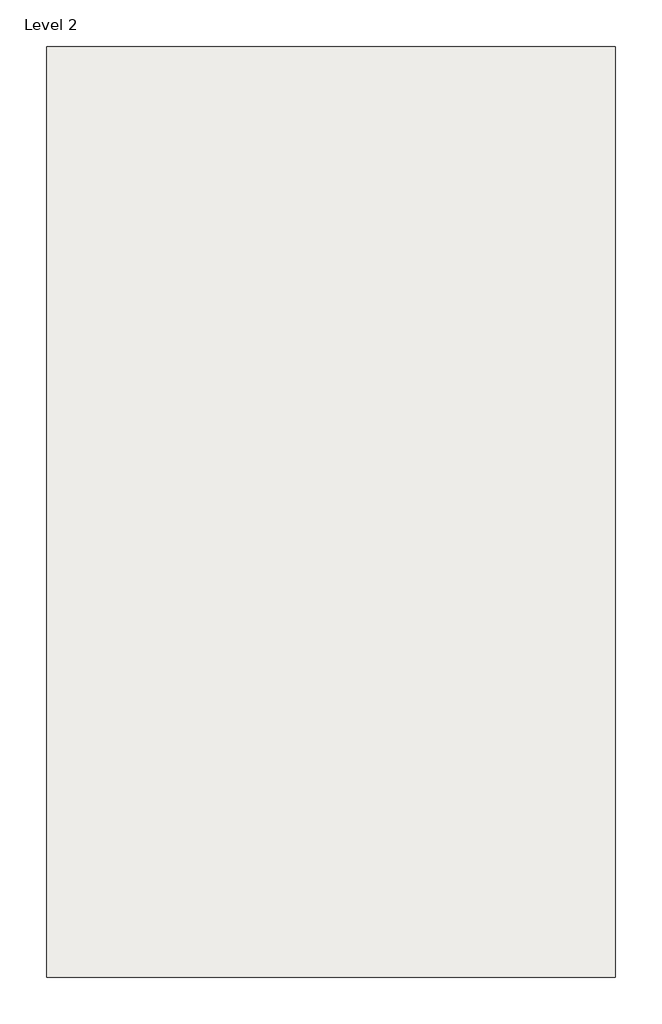
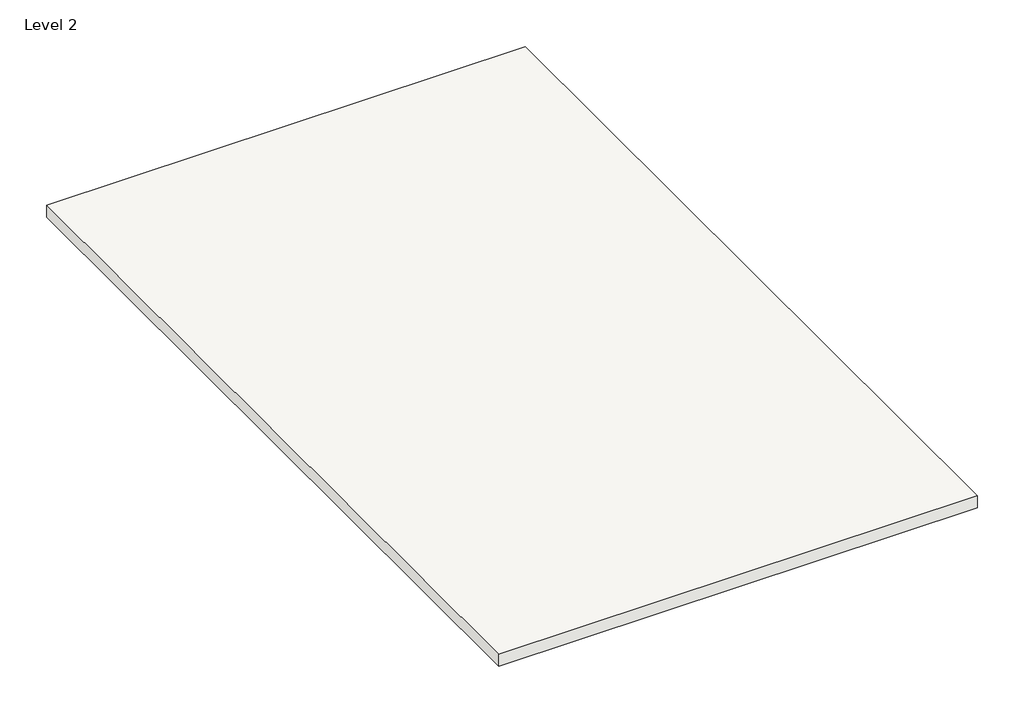
# One storey: 1 roof.
"""IFC4 building model written with IfcOpenShell, lengths in millimetres."""

from ifc_helpers import new_model, si_unit, frame, origin, place, context, project, spatial, polyline, outline, extrude, element, save

model = new_model("IFC4")

# Units and contexts
model_context = context("Model", 3, world=origin())
ifc_project = project(units=[si_unit("LENGTHUNIT", "METRE", prefix="MILLI")], contexts=[model_context])

# Site, building, storey
site = spatial("IfcSite", under=ifc_project)
building = spatial("IfcBuilding", under=site)
storey = spatial("IfcBuildingStorey", under=building, Name="Level 2", Elevation=3048.0)

# Roof
placement = place(None, origin())
element("IfcRoof", 1, ObjectType="Generic - 12\"", at=placement, inside=storey, context=model_context, shape_type="SweptSolid", body=[
    extrude(outline(polyline([(-12835.5505662, 12819.7742707), (-1354.7505662, 12819.7742707), (-1354.7505662, -5976.2257293), (-12835.5505662, -5976.2257293), (-12835.5505662, 12819.7742707)])), frame((0.0, 0.0, 3048.0), z_axis=(0.0, 0.0, 1.0), x_axis=(1.0, 0.0, 0.0)), (0.0, 0.0, 1.0), 304.8),
])

save(model, "model.ifc")

# Revit data of these elements
# Type "Generic - 12\""
#   Assembly Code = "B1020"
#   Layers, outside or top first: 1' - 0" "Brick, Soldier Course" (function 1)
# Element 1 (IfcRoof, "Generic - 12\"")
#   built-in parameter 1001705 = 11 (stored number, unit not read)
#   built-in parameter 1001710 = 33615
#   Phase Created = New Construction
#   Materials on its faces: "Brick, Soldier Course"
# Materials
#   "Brick, Soldier Course": class "Masonry", colour RGB 170 98 104, transparency 0, Description = "Common brick soldier coursed", Cost = 0
